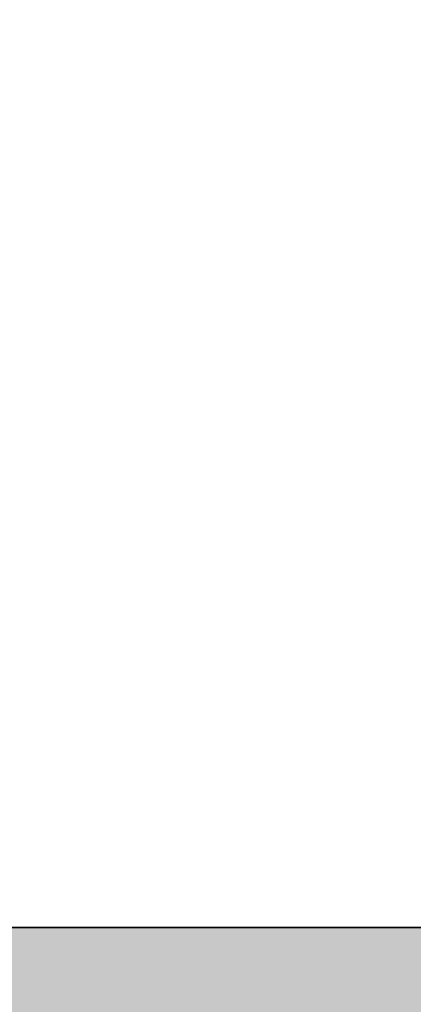
# Model space of a CAD drawing. Units: inches. Extents: x 2696 to 3240, y 1564 to 2310.
# Tile 29 of 76: x 3137.67 to 3142.32, y 1698.79 to 1710.43. Entities that reach past the tile are written whole.
import ezdxf

# ---------------------------------------------------------------- set-up
doc = ezdxf.new("R2010")
doc.units = ezdxf.units.IN
for name, color, linetype, lineweight in [('A-ANNO-DIMS', 3, 'Continuous', 18), ('A-WALL', 7, 'Continuous', 35), ('A-WALL-PATT', 9, 'Continuous', 13)]:
    doc.layers.add(name, color=color, linetype=linetype, lineweight=lineweight)
doc.styles.add('TIMES NEW', font='times.ttf')
doc.dimstyles.new('Siddhuu', dxfattribs={"dimtxt": 6, "dimasz": 2.5, "dimexe": 1.25, "dimexo": 0.625, "dimtad": 1, "dimdec": 1, "dimlunit": 4, "dimtxsty": 'TIMES NEW', "dimcen": 2.5, "dimclrd": 256, "dimclre": 1, "dimclrt": 7, "dimadec": 0, "dimazin": 0, "dimtfac": 1, "dimtdec": 1, "dimtmove": 0, "dimatfit": 3, "dimfxl": 1, "dimtolj": 1, "dimlwd": -1, "dimarcsym": 0})

# ---------------------------------------------------------------- blocks, each defined once
blk = doc.blocks.new('*D51')
at = {"layer": 'A-ANNO-DIMS', "color": 1, "lineweight": -2, "transparency": 16777216}
for p, q in [((3016.611, 1979.576), (3016.611, 1568.951)), ((3148.611, 1979.576), (3148.611, 1568.951))]:
    blk.add_line(p, q, dxfattribs=at)
at = {"layer": 'A-ANNO-DIMS', "transparency": 16777216}
blk.add_line((3019.111, 1570.201), (3146.111, 1570.201), dxfattribs=at)
for points in [[(3019.111, 1570.618), (3019.111, 1569.784), (3016.611, 1570.201)], [(3146.111, 1570.618), (3146.111, 1569.784), (3148.611, 1570.201)]]:
    blk.add_solid(points, dxfattribs=at)
at = {"layer": 'Defpoints', "color": 0, "transparency": 16777216}
for p in [(3016.611, 1980.201), (3148.611, 1980.201), (3148.611, 1570.201)]:
    blk.add_point(p, dxfattribs=at)
at = {"layer": 'A-ANNO-DIMS', "color": 7, "transparency": 16777216, "insert": (3082.611, 1573.878), "char_height": 6, "attachment_point": 5, "style": 'TIMES NEW'}
blk.add_mtext('\\A1;11\'-0"', dxfattribs=at)
blk = doc.blocks.new('*D56')
at = {"layer": 'A-ANNO-DIMS', "color": 1, "lineweight": -2, "transparency": 16777216}
for p, q in [((2966.334, 1884.201), (3235.861, 1884.201)), ((2966.334, 1665.201), (3235.861, 1665.201))]:
    blk.add_line(p, q, dxfattribs=at)
at = {"layer": 'A-ANNO-DIMS', "transparency": 16777216}
blk.add_line((3234.611, 1667.701), (3234.611, 1881.701), dxfattribs=at)
for points in [[(3234.195, 1881.701), (3235.028, 1881.701), (3234.611, 1884.201)], [(3234.195, 1667.701), (3235.028, 1667.701), (3234.611, 1665.201)]]:
    blk.add_solid(points, dxfattribs=at)
at = {"layer": 'Defpoints', "color": 0, "transparency": 16777216}
for p in [(2965.709, 1884.201), (3234.611, 1884.201), (2965.709, 1665.201)]:
    blk.add_point(p, dxfattribs=at)
at = {"layer": 'A-ANNO-DIMS', "color": 7, "transparency": 16777216, "insert": (3230.934, 1774.701), "char_height": 6, "attachment_point": 5, "rotation": 90, "style": 'TIMES NEW'}
blk.add_mtext('\\A1;18\'-3"', dxfattribs=at)

msp = doc.modelspace()

# ---------------------------------------------------------------- hatches: boundary and pattern name
at = {"layer": 'A-WALL-PATT', "transparency": 33554556}
h = msp.add_hatch(color=256, dxfattribs=at)
h.dxf.hatch_style = 1
h.paths.add_polyline_path([(2879.111, 2253.201), (2905.91, 2253.201), (2905.91, 2262.201), (2841.889, 2262.201), (2841.889, 2253.201), (2870.111, 2253.201), (2870.111, 2176.601), (2965.709, 2176.601), (2965.709, 2206.701), (2973.583, 2206.701), (2973.583, 2215.701), (2965.709, 2215.701), (2965.709, 2262.201), (2929.91, 2262.201), (2929.91, 2253.201), (2956.709, 2253.201), (2956.709, 2185.601), (2879.111, 2185.601)])
h.paths.add_polyline_path([(2782.834, 2262.201), (2745.611, 2262.201), (2745.611, 2228.729), (2754.611, 2228.729), (2754.611, 2253.201), (2782.834, 2253.201)])
h.paths.add_polyline_path([(2754.611, 2136.201), (2965.709, 2136.201), (2965.709, 2145.201), (2879.111, 2145.201), (2879.111, 2147.074), (2877.34, 2147.074), (2870.111, 2147.074), (2870.111, 2145.201), (2754.611, 2145.201), (2754.611, 2169.674), (2745.611, 2169.674), (2745.611, 2000.201), (2754.611, 2000.201), (2754.611, 2019.201), (2849.083, 2019.201), (2849.083, 2023.701), (2841.209, 2023.701), (2841.209, 2051.827), (2836.709, 2051.827), (2836.709, 2023.701), (2754.611, 2023.701), (2754.611, 2091.201), (2836.709, 2091.201), (2836.709, 2087.827), (2841.209, 2087.827), (2841.209, 2095.701), (2754.611, 2095.701)])
h.paths.add_polyline_path([(2965.709, 2136.201), (2956.709, 2136.201), (2956.709, 2023.701), (2885.083, 2023.701), (2885.083, 2019.201), (2956.709, 2019.201), (2956.709, 1950.575), (2965.709, 1950.575), (2965.709, 1980.201), (2973.583, 1980.201), (2973.583, 1989.201), (2965.709, 1989.201)])
h.paths.add_polyline_path([(2754.611, 1906.701), (2880.209, 1906.701), (2884.709, 1906.701), (2956.709, 1906.701), (2956.709, 1792.701), (2944.709, 1792.701), (2944.709, 1783.701), (2956.709, 1783.701), (2956.709, 1740.201), (2884.709, 1740.201), (2884.709, 1783.701), (2896.709, 1783.701), (2896.709, 1792.701), (2884.709, 1792.701), (2884.709, 1846.701), (2880.209, 1846.701), (2880.209, 1740.201), (2754.611, 1740.201), (2754.611, 1777.201), (2745.611, 1777.201), (2745.611, 1692.701), (2754.611, 1692.701), (2754.611, 1731.201), (2956.709, 1731.201), (2956.709, 1723.327), (2965.709, 1723.327), (2965.709, 1884.201), (2973.583, 1884.201), (2973.583, 1893.201), (2965.709, 1893.201), (2965.709, 1914.575), (2956.709, 1914.575), (2956.709, 1911.201), (2754.611, 1911.201), (2754.611, 1930.201), (2745.611, 1930.201), (2745.611, 1817.201), (2754.611, 1817.201), (2754.611, 1854.201), (2826.611, 1854.201), (2826.611, 1868.827), (2822.111, 1868.827), (2822.111, 1858.701), (2754.611, 1858.701)])
h.paths.add_polyline_path([(2965.709, 1656.201), (3008.237, 1656.201), (3008.237, 1665.201), (2965.709, 1665.201), (2965.709, 1693.327), (2956.709, 1693.327), (2956.709, 1686.201), (2934.583, 1686.201), (2934.583, 1681.701), (2956.709, 1681.701), (2956.709, 1614.201), (2896.709, 1614.201), (2896.709, 1681.701), (2904.583, 1681.701), (2904.583, 1686.201), (2892.209, 1686.201), (2892.209, 1614.201), (2858.41, 1614.201), (2858.41, 1605.201), (2965.709, 1605.201)])
h.paths.add_polyline_path([(2788.41, 1614.201), (2754.611, 1614.201), (2754.611, 1652.701), (2745.611, 1652.701), (2745.611, 1605.201), (2788.41, 1605.201)])
h.paths.add_polyline_path([(3199.611, 1633.048), (3190.611, 1633.048), (3190.611, 1614.201), (3082.611, 1614.201), (3082.611, 1665.201), (3070.237, 1665.201), (3070.237, 1656.201), (3078.111, 1656.201), (3078.111, 1605.201), (3199.611, 1605.201)])
h.paths.add_polyline_path([(3199.611, 1702.048), (3190.611, 1702.048), (3190.611, 1699.701), (3106.611, 1699.701), (3106.611, 1747.701), (3190.611, 1747.701), (3190.611, 1752.201), (3082.611, 1752.201), (3082.611, 1760.075), (3078.111, 1760.075), (3078.111, 1747.701), (3102.111, 1747.701), (3102.111, 1699.701), (3078.111, 1699.701), (3078.111, 1695.201), (3190.611, 1695.201), (3190.611, 1676.355), (3199.611, 1676.355)])
h.paths.add_polyline_path([(3199.611, 1783.201), (3190.611, 1783.201), (3190.611, 1745.355), (3199.611, 1745.355)])
h.paths.add_polyline_path([(3082.611, 1884.201), (3190.611, 1884.201), (3190.611, 1853.201), (3199.611, 1853.201), (3199.611, 1901.701), (3190.611, 1901.701), (3190.611, 1893.201), (3005.583, 1893.201), (3005.583, 1891.281), (3005.583, 1884.201), (3078.111, 1884.201), (3078.111, 1792.075), (3082.611, 1792.075)])
h.paths.add_polyline_path([(3199.611, 1994.701), (3190.611, 1994.701), (3190.611, 1989.201), (3073.709, 1989.201), (3073.709, 2034.201), (3069.209, 2034.201), (3069.209, 1989.201), (3005.583, 1989.201), (3005.583, 1980.201), (3190.611, 1980.201), (3190.611, 1971.701), (3199.611, 1971.701)])
h.paths.add_polyline_path([(3199.611, 2155.201), (3190.611, 2155.201), (3190.611, 2064.701), (3199.611, 2064.701)])
h.paths.add_polyline_path([(3190.611, 2074.701), (3106.611, 2074.701), (3106.611, 2122.701), (3190.611, 2122.701), (3190.611, 2127.201), (3082.709, 2127.201), (3082.709, 2135.075), (3073.709, 2135.075), (3073.709, 2122.701), (3102.111, 2122.701), (3102.111, 2074.701), (3069.209, 2074.701), (3069.209, 2070.201), (3190.611, 2070.201)])
h.paths.add_polyline_path([(3082.709, 2253.201), (3190.611, 2253.201), (3190.611, 2225.201), (3199.611, 2225.201), (3199.611, 2262.201), (3073.709, 2262.201), (3073.709, 2215.701), (3035.583, 2215.701), (3035.583, 2206.701), (3073.709, 2206.701), (3073.709, 2171.075), (3082.709, 2171.075)])

# ---------------------------------------------------------------- linework, layer by layer
at = {"layer": 'A-WALL'}
msp.add_line((3106.611, 1699.701), (3190.611, 1699.701), dxfattribs=at)

# ---------------------------------------------------------------- dimensions: what is measured, and where the dimension line sits
at = {"layer": 'A-ANNO-DIMS'}
dim = msp.add_linear_dim(base=(3148.611, 1570.201), p1=(3016.611, 1980.201), p2=(3148.611, 1980.201), dimstyle='Siddhuu', override={"dimdec": 1, "dimlfac": 1, "dimrnd": 0, "dimzin": 1, "dimdsep": 46, "dimlunit": 4, "dimfrac": 2}, dxfattribs=at)
dim.commit()
dim.dimension.update_dxf_attribs({"geometry": '*D51', "text_midpoint": (3082.611, 1573.878)})
dim = msp.add_linear_dim(base=(3234.611, 1884.201), p1=(2965.709, 1665.201), p2=(2965.709, 1884.201), angle=90, dimstyle='Siddhuu', override={"dimdec": 1, "dimlfac": 1, "dimrnd": 0, "dimzin": 1, "dimdsep": 46, "dimlunit": 4, "dimfrac": 2}, dxfattribs=at)
dim.commit()
dim.dimension.update_dxf_attribs({"geometry": '*D56', "text_midpoint": (3230.934, 1774.701)})

doc.saveas('drawing.dxf')
